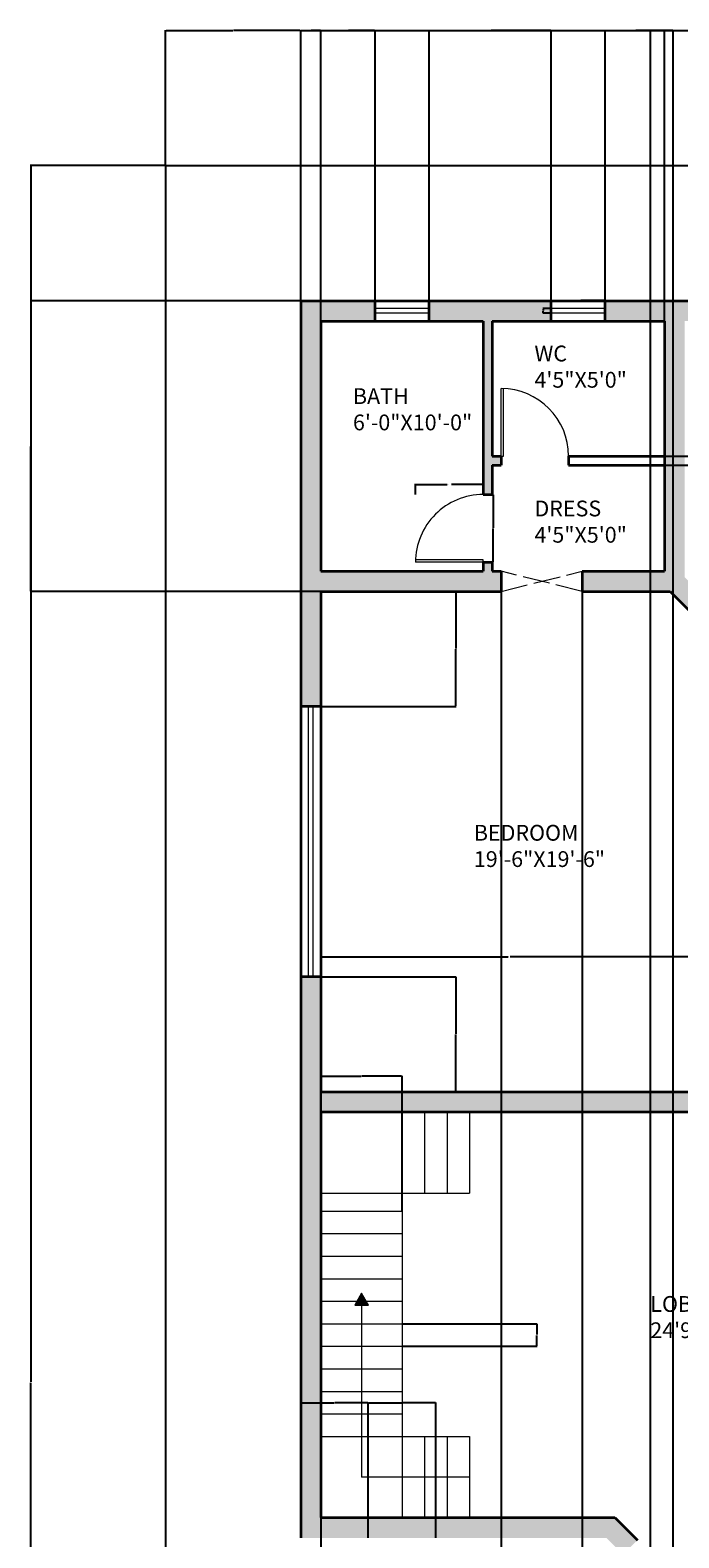
# Model space of a CAD drawing. Units: inches. Extents: x 1516 to 2236, y 3034 to 4235.
# Tile 2 of 3: x 1516 to 1804, y 3566 to 4235. Entities that reach past the tile are written whole.
import ezdxf

# ---------------------------------------------------------------- set-up
doc = ezdxf.new("R2010")
doc.units = ezdxf.units.IN
doc.linetypes.add('ACAD_ISO02W100', pattern=[15, 12, -3])
for name, color, linetype, lineweight in [('A-ANNO-DIMS', 2, 'Continuous', 18), ('A-ANNO-SYMB', 7, 'Continuous', 18), ('A-AREA-IDEN', 7, 'Continuous', 18), ('A-DOOR', 3, 'Continuous', 18), ('A-FLOR-STRS', 7, 'Continuous', 18), ('A-GLAZ', 4, 'Continuous', 18), ('A-WALL', 7, 'Continuous', 35), ('A-WALL-OVHD', 8, 'ACAD_ISO02W100', 13), ('A-WALL-PATT', 252, 'Continuous', 13), ('C-PROP', 8, 'Continuous', 25)]:
    doc.layers.add(name, color=color, linetype=linetype, lineweight=lineweight)
doc.styles.get("Standard").update_dxf_attribs({"font": 'arial.ttf'})
doc.dimstyles.get("Standard").update_dxf_attribs({"dimtxt": 0.18, "dimasz": 0.18, "dimexe": 0.18, "dimexo": 0.0625, "dimgap": 0.09, "dimtad": 0, "dimtih": 1, "dimtoh": 1, "dimdec": 4, "dimzin": 0, "dimdsep": 46, "dimtxsty": 'Standard', "dimcen": 0.09, "dimadec": 0, "dimazin": 0, "dimtfac": 1, "dimtdec": 4, "dimtofl": 0, "dimtmove": 0, "dimatfit": 3, "dimfxl": 1, "dimtolj": 1, "dimtzin": 0, "dimarcsym": 0})

# ---------------------------------------------------------------- blocks, each defined once
blk = doc.blocks.new('DOOR-30IN-SWING')
for p, q in [((0, 0), (0, 30)), ((1, 0), (1, 29.98)), ((0, 0), (1, 0))]:
    blk.add_line(p, q)
blk.add_arc((0, 0), 30, 0, 90)
blk = doc.blocks.new('WIN-120IN-GLASS')
for p, q in [((120, 2), (0, 2)), ((120, 0), (0, 0))]:
    blk.add_line(p, q)
blk = doc.blocks.new('WIN-24IN-GLASS')
for p, q in [((24, 2), (0, 2)), ((24, 0), (0, 0))]:
    blk.add_line(p, q)
blk = doc.blocks.new('*D8')
at = {"layer": 'A-ANNO-DIMS', "color": 0, "lineweight": -2, "transparency": 16777216}
for p, q in [((1747.26, 4111.08), (1747.26, 4114.8)), ((1747.44, 4114.62), (1758.15, 4114.62)), ((1771.08, 4114.62), (1760.38, 4114.62)), ((1771.26, 4111.08), (1771.26, 4114.8))]:
    blk.add_line(p, q, dxfattribs=at)
at = {"layer": 'A-ANNO-DIMS', "color": 0, "transparency": 16777216}
for points in [[(1747.44, 4114.65), (1747.44, 4114.59), (1747.26, 4114.62)], [(1771.08, 4114.65), (1771.08, 4114.59), (1771.26, 4114.62)]]:
    blk.add_solid(points, dxfattribs=at)
at = {"layer": 'Defpoints', "color": 0, "transparency": 16777216}
for p in [(1747.26, 4111.02), (1771.26, 4114.62), (1771.26, 4111.02)]:
    blk.add_point(p, dxfattribs=at)
at = {"layer": 'A-ANNO-DIMS', "color": 0, "transparency": 16777216, "insert": (1759.26, 4114.62), "char_height": 0.18, "attachment_point": 5}
blk.add_mtext('\\A1;WINDOW 24 TYP.', dxfattribs=at)
blk = doc.blocks.new('*D9')
at = {"layer": 'A-ANNO-DIMS', "color": 0, "lineweight": -2, "transparency": 16777216}
for p, q in [((1747.2, 4111.02), (1743.48, 4111.02)), ((1747.2, 4109.02), (1743.48, 4109.02)), ((1743.66, 4110.84), (1743.66, 4110.2)), ((1743.66, 4109.2), (1743.66, 4109.84))]:
    blk.add_line(p, q, dxfattribs=at)
at = {"layer": 'A-ANNO-DIMS', "color": 0, "transparency": 16777216}
for points in [[(1743.63, 4110.84), (1743.69, 4110.84), (1743.66, 4111.02)], [(1743.63, 4109.2), (1743.69, 4109.2), (1743.66, 4109.02)]]:
    blk.add_solid(points, dxfattribs=at)
at = {"layer": 'Defpoints', "color": 0, "transparency": 16777216}
for p in [(1743.66, 4111.02), (1747.26, 4111.02), (1747.26, 4109.02)]:
    blk.add_point(p, dxfattribs=at)
at = {"layer": 'A-ANNO-DIMS', "color": 0, "transparency": 16777216, "insert": (1743.66, 4110.02), "char_height": 0.18, "attachment_point": 5}
blk.add_mtext('\\A1;2 TYP.', dxfattribs=at)
blk = doc.blocks.new('*D14')
at = {"layer": 'A-ANNO-DIMS', "color": 0, "lineweight": -2, "transparency": 16777216}
for p, q in [((1687.01, 4028.58), (1687.01, 4033.2)), ((1687.19, 4033.02), (1701.08, 4033.02)), ((1716.83, 4033.02), (1702.95, 4033.02)), ((1717.01, 4028.58), (1717.01, 4033.2))]:
    blk.add_line(p, q, dxfattribs=at)
at = {"layer": 'A-ANNO-DIMS', "color": 0, "transparency": 16777216}
for points in [[(1687.19, 4033.05), (1687.19, 4032.99), (1687.01, 4033.02)], [(1716.83, 4033.05), (1716.83, 4032.99), (1717.01, 4033.02)]]:
    blk.add_solid(points, dxfattribs=at)
at = {"layer": 'Defpoints', "color": 0, "transparency": 16777216}
for p in [(1687.01, 4033.02), (1687.01, 4028.52), (1717.01, 4028.52)]:
    blk.add_point(p, dxfattribs=at)
at = {"layer": 'A-ANNO-DIMS', "color": 0, "transparency": 16777216, "insert": (1702.01, 4033.02), "char_height": 0.18, "attachment_point": 5}
blk.add_mtext('\\A1;DOOR 30 TYP.', dxfattribs=at)
blk = doc.blocks.new('*D15')
at = {"layer": 'A-ANNO-DIMS', "color": 0, "lineweight": -2, "transparency": 16777216}
for p, q in [((1717.08, 4028.52), (1721.69, 4028.52)), ((1721.51, 4028.34), (1721.51, 4013.7)), ((1721.51, 3998.7), (1721.51, 4013.34)), ((1717.08, 3998.52), (1721.69, 3998.52))]:
    blk.add_line(p, q, dxfattribs=at)
at = {"layer": 'A-ANNO-DIMS', "color": 0, "transparency": 16777216}
for points in [[(1721.48, 4028.34), (1721.54, 4028.34), (1721.51, 4028.52)], [(1721.48, 3998.7), (1721.54, 3998.7), (1721.51, 3998.52)]]:
    blk.add_solid(points, dxfattribs=at)
at = {"layer": 'Defpoints', "color": 0, "transparency": 16777216}
for p in [(1717.01, 4028.52), (1721.51, 4028.52), (1717.01, 3998.52)]:
    blk.add_point(p, dxfattribs=at)
at = {"layer": 'A-ANNO-DIMS', "color": 0, "transparency": 16777216, "insert": (1721.51, 4013.52), "char_height": 0.18, "attachment_point": 5}
blk.add_mtext('\\A1;30 TYP.', dxfattribs=at)
blk = doc.blocks.new('*D17')
at = {"layer": 'A-ANNO-DIMS', "color": 0, "lineweight": -2, "transparency": 16777216}
for p, q in [((1575.95, 4174.52), (1515.93, 4174.52)), ((1516.11, 4174.34), (1516.11, 3634.7)), ((1516.11, 3094.7), (1516.11, 3634.34)), ((1575.95, 3094.52), (1515.93, 3094.52))]:
    blk.add_line(p, q, dxfattribs=at)
at = {"layer": 'A-ANNO-DIMS', "color": 0, "transparency": 16777216}
for points in [[(1516.08, 4174.34), (1516.14, 4174.34), (1516.11, 4174.52)], [(1516.08, 3094.7), (1516.14, 3094.7), (1516.11, 3094.52)]]:
    blk.add_solid(points, dxfattribs=at)
at = {"layer": 'Defpoints', "color": 0, "transparency": 16777216}
for p in [(1516.11, 4174.52), (1576.01, 4174.52), (1576.01, 3094.52)]:
    blk.add_point(p, dxfattribs=at)
at = {"layer": 'A-ANNO-DIMS', "color": 0, "transparency": 16777216, "insert": (1516.11, 3634.52), "char_height": 0.18, "attachment_point": 5}
blk.add_mtext('\\A1;1080', dxfattribs=at)
blk = doc.blocks.new('*D18')
at = {"layer": 'A-ANNO-DIMS', "color": 0, "lineweight": -2, "transparency": 16777216}
for p, q in [((1576.01, 4174.58), (1576.01, 4234.6)), ((1576.19, 4234.42), (1605.8, 4234.42)), ((1635.83, 4234.42), (1606.23, 4234.42)), ((1636.01, 4114.58), (1636.01, 4234.6))]:
    blk.add_line(p, q, dxfattribs=at)
at = {"layer": 'A-ANNO-DIMS', "color": 0, "transparency": 16777216}
for points in [[(1576.19, 4234.45), (1576.19, 4234.39), (1576.01, 4234.42)], [(1635.83, 4234.45), (1635.83, 4234.39), (1636.01, 4234.42)]]:
    blk.add_solid(points, dxfattribs=at)
at = {"layer": 'Defpoints', "color": 0, "transparency": 16777216}
for p in [(1636.01, 4234.42), (1576.01, 4174.52), (1636.01, 4114.52)]:
    blk.add_point(p, dxfattribs=at)
at = {"layer": 'A-ANNO-DIMS', "color": 0, "transparency": 16777216, "insert": (1606.01, 4234.42), "char_height": 0.18, "attachment_point": 5}
blk.add_mtext('\\A1;60', dxfattribs=at)
blk = doc.blocks.new('*D19')
at = {"layer": 'A-ANNO-DIMS', "color": 0, "lineweight": -2, "transparency": 16777216}
for p, q in [((1636.01, 4114.58), (1636.01, 4234.6)), ((1636.19, 4234.42), (1875.37, 4234.42)), ((2115.33, 4234.42), (1876.16, 4234.42)), ((2115.51, 4114.58), (2115.51, 4234.6))]:
    blk.add_line(p, q, dxfattribs=at)
at = {"layer": 'A-ANNO-DIMS', "color": 0, "transparency": 16777216}
for points in [[(1636.19, 4234.45), (1636.19, 4234.39), (1636.01, 4234.42)], [(2115.33, 4234.45), (2115.33, 4234.39), (2115.51, 4234.42)]]:
    blk.add_solid(points, dxfattribs=at)
at = {"layer": 'Defpoints', "color": 0, "transparency": 16777216}
for p in [(2115.51, 4234.42), (1636.01, 4114.52), (2115.51, 4114.52)]:
    blk.add_point(p, dxfattribs=at)
at = {"layer": 'A-ANNO-DIMS', "color": 0, "transparency": 16777216, "insert": (1875.76, 4234.42), "char_height": 0.18, "attachment_point": 5}
blk.add_mtext('\\A1;479.5', dxfattribs=at)
blk = doc.blocks.new('*D29')
at = {"layer": 'A-ANNO-DIMS', "color": 0, "lineweight": -2, "transparency": 16777216}
for p, q in [((1645.08, 3985.52), (1705.09, 3985.52)), ((1704.91, 3985.34), (1704.91, 3960.2)), ((1704.91, 3934.7), (1704.91, 3959.84)), ((1645.08, 3934.52), (1705.09, 3934.52))]:
    blk.add_line(p, q, dxfattribs=at)
at = {"layer": 'A-ANNO-DIMS', "color": 0, "transparency": 16777216}
for points in [[(1704.88, 3985.34), (1704.94, 3985.34), (1704.91, 3985.52)], [(1704.88, 3934.7), (1704.94, 3934.7), (1704.91, 3934.52)]]:
    blk.add_solid(points, dxfattribs=at)
at = {"layer": 'Defpoints', "color": 0, "transparency": 16777216}
for p in [(1645.01, 3985.52), (1645.01, 3934.52), (1704.91, 3934.52)]:
    blk.add_point(p, dxfattribs=at)
at = {"layer": 'A-ANNO-DIMS', "color": 0, "transparency": 16777216, "insert": (1704.91, 3960.02), "char_height": 0.18, "attachment_point": 5}
blk.add_mtext('\\A1;51', dxfattribs=at)
blk = doc.blocks.new('*D30')
at = {"layer": 'A-ANNO-DIMS', "color": 0, "lineweight": -2, "transparency": 16777216}
for p, q in [((1645.08, 3814.52), (1705.09, 3814.52)), ((1704.91, 3814.34), (1704.91, 3789.2)), ((1704.91, 3763.7), (1704.91, 3788.84)), ((1645.08, 3763.52), (1705.09, 3763.52))]:
    blk.add_line(p, q, dxfattribs=at)
at = {"layer": 'A-ANNO-DIMS', "color": 0, "transparency": 16777216}
for points in [[(1704.88, 3814.34), (1704.94, 3814.34), (1704.91, 3814.52)], [(1704.88, 3763.7), (1704.94, 3763.7), (1704.91, 3763.52)]]:
    blk.add_solid(points, dxfattribs=at)
at = {"layer": 'Defpoints', "color": 0, "transparency": 16777216}
for p in [(1645.01, 3814.52), (1645.01, 3763.52), (1704.91, 3763.52)]:
    blk.add_point(p, dxfattribs=at)
at = {"layer": 'A-ANNO-DIMS', "color": 0, "transparency": 16777216, "insert": (1704.91, 3789.02), "char_height": 0.18, "attachment_point": 5}
blk.add_mtext('\\A1;51', dxfattribs=at)
blk = doc.blocks.new('*D31')
at = {"layer": 'A-ANNO-DIMS', "color": 0, "lineweight": -2, "transparency": 16777216}
for p, q in [((1645.01, 3763.58), (1645.01, 3823.6)), ((1645.19, 3823.42), (1728.13, 3823.42)), ((1811.97, 3823.42), (1729.04, 3823.42)), ((1812.15, 3763.58), (1812.15, 3823.6))]:
    blk.add_line(p, q, dxfattribs=at)
at = {"layer": 'A-ANNO-DIMS', "color": 0, "transparency": 16777216}
for points in [[(1645.19, 3823.45), (1645.19, 3823.39), (1645.01, 3823.42)], [(1811.97, 3823.45), (1811.97, 3823.39), (1812.15, 3823.42)]]:
    blk.add_solid(points, dxfattribs=at)
at = {"layer": 'Defpoints', "color": 0, "transparency": 16777216}
for p in [(1812.15, 3823.42), (1645.01, 3763.52), (1812.15, 3763.52)]:
    blk.add_point(p, dxfattribs=at)
at = {"layer": 'A-ANNO-DIMS', "color": 0, "transparency": 16777216, "insert": (1728.58, 3823.42), "char_height": 0.18, "attachment_point": 5}
blk.add_mtext('\\A1;167.14', dxfattribs=at)
blk = doc.blocks.new('*D32')
at = {"layer": 'A-ANNO-DIMS', "color": 0, "lineweight": -2, "transparency": 16777216}
for p, q in [((1636.01, 3565.58), (1636.01, 3625.6)), ((1636.19, 3625.42), (1650.8, 3625.42)), ((1665.83, 3625.42), (1651.23, 3625.42)), ((1666.01, 3565.58), (1666.01, 3625.6))]:
    blk.add_line(p, q, dxfattribs=at)
at = {"layer": 'A-ANNO-DIMS', "color": 0, "transparency": 16777216}
for points in [[(1636.19, 3625.45), (1636.19, 3625.39), (1636.01, 3625.42)], [(1665.83, 3625.45), (1665.83, 3625.39), (1666.01, 3625.42)]]:
    blk.add_solid(points, dxfattribs=at)
at = {"layer": 'Defpoints', "color": 0, "transparency": 16777216}
for p in [(1666.01, 3625.42), (1636.01, 3565.52), (1666.01, 3565.52)]:
    blk.add_point(p, dxfattribs=at)
at = {"layer": 'A-ANNO-DIMS', "color": 0, "transparency": 16777216, "insert": (1651.01, 3625.42), "char_height": 0.18, "attachment_point": 5}
blk.add_mtext('\\A1;30', dxfattribs=at)
blk = doc.blocks.new('*D33')
at = {"layer": 'A-ANNO-DIMS', "color": 0, "lineweight": -2, "transparency": 16777216}
for p, q in [((1666.01, 3565.58), (1666.01, 3625.6)), ((1666.19, 3625.42), (1680.8, 3625.42)), ((1695.83, 3625.42), (1681.23, 3625.42)), ((1696.01, 3565.58), (1696.01, 3625.6))]:
    blk.add_line(p, q, dxfattribs=at)
at = {"layer": 'A-ANNO-DIMS', "color": 0, "transparency": 16777216}
for points in [[(1666.19, 3625.45), (1666.19, 3625.39), (1666.01, 3625.42)], [(1695.83, 3625.45), (1695.83, 3625.39), (1696.01, 3625.42)]]:
    blk.add_solid(points, dxfattribs=at)
at = {"layer": 'Defpoints', "color": 0, "transparency": 16777216}
for p in [(1696.01, 3625.42), (1666.01, 3565.52), (1696.01, 3565.52)]:
    blk.add_point(p, dxfattribs=at)
at = {"layer": 'A-ANNO-DIMS', "color": 0, "transparency": 16777216, "insert": (1681.01, 3625.42), "char_height": 0.18, "attachment_point": 5}
blk.add_mtext('\\A1;30', dxfattribs=at)
blk = doc.blocks.new('*D34')
at = {"layer": 'A-ANNO-DIMS', "color": 0, "lineweight": -2, "transparency": 16777216}
for p, q in [((1645.01, 4105.58), (1645.01, 4234.6)), ((1645.19, 4234.42), (1656.79, 4234.42)), ((1668.83, 4234.42), (1657.23, 4234.42)), ((1669.01, 4114.58), (1669.01, 4234.6))]:
    blk.add_line(p, q, dxfattribs=at)
at = {"layer": 'A-ANNO-DIMS', "color": 0, "transparency": 16777216}
for points in [[(1645.19, 4234.45), (1645.19, 4234.39), (1645.01, 4234.42)], [(1668.83, 4234.45), (1668.83, 4234.39), (1669.01, 4234.42)]]:
    blk.add_solid(points, dxfattribs=at)
at = {"layer": 'Defpoints', "color": 0, "transparency": 16777216}
for p in [(1669.01, 4234.42), (1669.01, 4114.52), (1645.01, 4105.52)]:
    blk.add_point(p, dxfattribs=at)
at = {"layer": 'A-ANNO-DIMS', "color": 0, "transparency": 16777216, "insert": (1657.01, 4234.42), "char_height": 0.18, "attachment_point": 5}
blk.add_mtext('\\A1;24', dxfattribs=at)
blk = doc.blocks.new('*D35')
at = {"layer": 'A-ANNO-DIMS', "color": 0, "lineweight": -2, "transparency": 16777216}
for p, q in [((1693.01, 4114.58), (1693.01, 4234.6)), ((1693.19, 4234.42), (1719.74, 4234.42)), ((1747.08, 4234.42), (1720.53, 4234.42)), ((1747.26, 4114.58), (1747.26, 4234.6))]:
    blk.add_line(p, q, dxfattribs=at)
at = {"layer": 'A-ANNO-DIMS', "color": 0, "transparency": 16777216}
for points in [[(1693.19, 4234.45), (1693.19, 4234.39), (1693.01, 4234.42)], [(1747.08, 4234.45), (1747.08, 4234.39), (1747.26, 4234.42)]]:
    blk.add_solid(points, dxfattribs=at)
at = {"layer": 'Defpoints', "color": 0, "transparency": 16777216}
for p in [(1747.26, 4234.42), (1693.01, 4114.52), (1747.26, 4114.52)]:
    blk.add_point(p, dxfattribs=at)
at = {"layer": 'A-ANNO-DIMS', "color": 0, "transparency": 16777216, "insert": (1720.14, 4234.42), "char_height": 0.18, "attachment_point": 5}
blk.add_mtext('\\A1;54.25', dxfattribs=at)
blk = doc.blocks.new('*D36')
at = {"layer": 'A-ANNO-DIMS', "color": 0, "lineweight": -2, "transparency": 16777216}
for p, q in [((1771.26, 4114.58), (1771.26, 4234.6)), ((1771.44, 4234.42), (1783.99, 4234.42)), ((1797.33, 4234.42), (1784.79, 4234.42)), ((1797.51, 4105.58), (1797.51, 4234.6))]:
    blk.add_line(p, q, dxfattribs=at)
at = {"layer": 'A-ANNO-DIMS', "color": 0, "transparency": 16777216}
for points in [[(1771.44, 4234.45), (1771.44, 4234.39), (1771.26, 4234.42)], [(1797.33, 4234.45), (1797.33, 4234.39), (1797.51, 4234.42)]]:
    blk.add_solid(points, dxfattribs=at)
at = {"layer": 'Defpoints', "color": 0, "transparency": 16777216}
for p in [(1797.51, 4234.42), (1771.26, 4114.52), (1797.51, 4105.52)]:
    blk.add_point(p, dxfattribs=at)
at = {"layer": 'A-ANNO-DIMS', "color": 0, "transparency": 16777216, "insert": (1784.39, 4234.42), "char_height": 0.18, "attachment_point": 5}
blk.add_mtext('\\A1;26.25', dxfattribs=at)
blk = doc.blocks.new('*D37')
at = {"layer": 'A-ANNO-DIMS', "color": 0, "lineweight": -2, "transparency": 16777216}
for p, q in [((1645.01, 3985.46), (1645.01, 3034.44)), ((1725.01, 3985.46), (1725.01, 3034.44)), ((1645.19, 3034.62), (1684.8, 3034.62)), ((1724.83, 3034.62), (1685.23, 3034.62))]:
    blk.add_line(p, q, dxfattribs=at)
at = {"layer": 'A-ANNO-DIMS', "color": 0, "transparency": 16777216}
for points in [[(1645.19, 3034.65), (1645.19, 3034.59), (1645.01, 3034.62)], [(1724.83, 3034.65), (1724.83, 3034.59), (1725.01, 3034.62)]]:
    blk.add_solid(points, dxfattribs=at)
at = {"layer": 'Defpoints', "color": 0, "transparency": 16777216}
for p in [(1645.01, 3985.52), (1725.01, 3985.52), (1725.01, 3034.62)]:
    blk.add_point(p, dxfattribs=at)
at = {"layer": 'A-ANNO-DIMS', "color": 0, "transparency": 16777216, "insert": (1685.01, 3034.62), "char_height": 0.18, "attachment_point": 5}
blk.add_mtext('\\A1;80', dxfattribs=at)
blk = doc.blocks.new('*D38')
at = {"layer": 'A-ANNO-DIMS', "color": 0, "lineweight": -2, "transparency": 16777216}
for p, q in [((1725.01, 3985.46), (1725.01, 3034.44)), ((1761.01, 3985.46), (1761.01, 3034.44)), ((1725.19, 3034.62), (1742.8, 3034.62)), ((1760.83, 3034.62), (1743.23, 3034.62))]:
    blk.add_line(p, q, dxfattribs=at)
at = {"layer": 'A-ANNO-DIMS', "color": 0, "transparency": 16777216}
for points in [[(1725.19, 3034.65), (1725.19, 3034.59), (1725.01, 3034.62)], [(1760.83, 3034.65), (1760.83, 3034.59), (1761.01, 3034.62)]]:
    blk.add_solid(points, dxfattribs=at)
at = {"layer": 'Defpoints', "color": 0, "transparency": 16777216}
for p in [(1725.01, 3985.52), (1761.01, 3985.52), (1761.01, 3034.62)]:
    blk.add_point(p, dxfattribs=at)
at = {"layer": 'A-ANNO-DIMS', "color": 0, "transparency": 16777216, "insert": (1743.01, 3034.62), "char_height": 0.18, "attachment_point": 5}
blk.add_mtext('\\A1;36', dxfattribs=at)
blk = doc.blocks.new('*D39')
at = {"layer": 'A-ANNO-DIMS', "color": 0, "lineweight": -2, "transparency": 16777216}
for p, q in [((1797.57679, 4045.522053), (2236.09429, 4045.522053)), ((1797.57679, 4041.522053), (2236.09429, 4041.522053)), ((2235.91429, 4045.342053), (2235.91429, 4043.702053)), ((2235.91429, 4041.702053), (2235.91429, 4043.342053))]:
    blk.add_line(p, q, dxfattribs=at)
at = {"layer": 'A-ANNO-DIMS', "color": 0, "transparency": 16777216}
for points in [[(2235.88429, 4045.342053), (2235.94429, 4045.342053), (2235.91429, 4045.522053)], [(2235.88429, 4041.702053), (2235.94429, 4041.702053), (2235.91429, 4041.522053)]]:
    blk.add_solid(points, dxfattribs=at)
at = {"layer": 'Defpoints', "color": 0, "transparency": 16777216}
for p in [(1797.51429, 4045.522053), (1797.51429, 4041.522053), (2235.91429, 4045.522053)]:
    blk.add_point(p, dxfattribs=at)
at = {"layer": 'A-ANNO-DIMS', "color": 0, "transparency": 16777216, "insert": (2235.91429, 4043.522053), "char_height": 0.18, "attachment_point": 5}
blk.add_mtext('\\A1;4', dxfattribs=at)
blk = doc.blocks.new('*D40')
at = {"layer": 'A-ANNO-DIMS', "color": 0, "lineweight": -2, "transparency": 16777216}
for p, q in [((1635.95, 4114.52), (1515.93, 4114.52)), ((1516.11, 4114.34), (1516.11, 4050.2)), ((1516.11, 3985.7), (1516.11, 4049.84)), ((1644.95, 3985.52), (1515.93, 3985.52))]:
    blk.add_line(p, q, dxfattribs=at)
at = {"layer": 'A-ANNO-DIMS', "color": 0, "transparency": 16777216}
for points in [[(1516.08, 4114.34), (1516.14, 4114.34), (1516.11, 4114.52)], [(1516.08, 3985.7), (1516.14, 3985.7), (1516.11, 3985.52)]]:
    blk.add_solid(points, dxfattribs=at)
at = {"layer": 'Defpoints', "color": 0, "transparency": 16777216}
for p in [(1636.01, 4114.52), (1516.11, 3985.52), (1645.01, 3985.52)]:
    blk.add_point(p, dxfattribs=at)
at = {"layer": 'A-ANNO-DIMS', "color": 0, "transparency": 16777216, "insert": (1516.11, 4050.02), "char_height": 0.18, "attachment_point": 5}
blk.add_mtext('\\A1;129', dxfattribs=at)
blk = doc.blocks.new('*D41')
at = {"layer": 'A-ANNO-DIMS', "color": 0, "lineweight": -2, "transparency": 16777216}
for p, q in [((1636.01, 4114.58), (1636.01, 4234.6)), ((1636.19, 4234.42), (1640.37, 4234.42)), ((1644.83, 4234.42), (1640.66, 4234.42)), ((1645.01, 4105.58), (1645.01, 4234.6))]:
    blk.add_line(p, q, dxfattribs=at)
at = {"layer": 'A-ANNO-DIMS', "color": 0, "transparency": 16777216}
for points in [[(1636.19, 4234.45), (1636.19, 4234.39), (1636.01, 4234.42)], [(1644.83, 4234.45), (1644.83, 4234.39), (1645.01, 4234.42)]]:
    blk.add_solid(points, dxfattribs=at)
at = {"layer": 'Defpoints', "color": 0, "transparency": 16777216}
for p in [(1645.01, 4234.42), (1636.01, 4114.52), (1645.01, 4105.52)]:
    blk.add_point(p, dxfattribs=at)
at = {"layer": 'A-ANNO-DIMS', "color": 0, "transparency": 16777216, "insert": (1640.51, 4234.42), "char_height": 0.18, "attachment_point": 5}
blk.add_mtext('\\A1;9', dxfattribs=at)
blk = doc.blocks.new('*D49')
at = {"layer": 'A-ANNO-DIMS', "color": 0, "lineweight": -2, "transparency": 16777216}
for p, q in [((1791.4, 3240.97), (1791.4, 4234.6)), ((1791.58, 4234.42), (1796.19, 4234.42)), ((1801.22, 4234.42), (1796.61, 4234.42)), ((1801.4, 3240.97), (1801.4, 4234.6))]:
    blk.add_line(p, q, dxfattribs=at)
at = {"layer": 'A-ANNO-DIMS', "color": 0, "transparency": 16777216}
for points in [[(1791.58, 4234.45), (1791.58, 4234.39), (1791.4, 4234.42)], [(1801.22, 4234.45), (1801.22, 4234.39), (1801.4, 4234.42)]]:
    blk.add_solid(points, dxfattribs=at)
at = {"layer": 'Defpoints', "color": 0, "transparency": 16777216}
for p in [(1801.4, 4234.42), (1791.4, 3240.91), (1801.4, 3240.91)]:
    blk.add_point(p, dxfattribs=at)
at = {"layer": 'A-ANNO-DIMS', "color": 0, "transparency": 16777216, "insert": (1796.4, 4234.42), "char_height": 0.18, "attachment_point": 5}
blk.add_mtext('\\A1;10', dxfattribs=at)
blk = doc.blocks.new('*D54')
at = {"layer": 'A-ANNO-DIMS', "color": 0, "lineweight": -2, "transparency": 16777216}
for p, q in [((1645.01, 3710.58), (1645.01, 3770.6)), ((1645.19, 3770.42), (1662.8, 3770.42)), ((1680.83, 3770.42), (1663.23, 3770.42)), ((1681.01, 3710.58), (1681.01, 3770.6))]:
    blk.add_line(p, q, dxfattribs=at)
at = {"layer": 'A-ANNO-DIMS', "color": 0, "transparency": 16777216}
for points in [[(1645.19, 3770.45), (1645.19, 3770.39), (1645.01, 3770.42)], [(1680.83, 3770.45), (1680.83, 3770.39), (1681.01, 3770.42)]]:
    blk.add_solid(points, dxfattribs=at)
at = {"layer": 'Defpoints', "color": 0, "transparency": 16777216}
for p in [(1681.01, 3770.42), (1645.01, 3710.52), (1681.01, 3710.52)]:
    blk.add_point(p, dxfattribs=at)
at = {"layer": 'A-ANNO-DIMS', "color": 0, "transparency": 16777216, "insert": (1663.01, 3770.42), "char_height": 0.18, "attachment_point": 5}
blk.add_mtext('\\A1;36', dxfattribs=at)
blk = doc.blocks.new('*D55')
at = {"layer": 'A-ANNO-DIMS', "color": 0, "lineweight": -2, "transparency": 16777216}
for p, q in [((1681.08, 3660.52), (1741.09, 3660.52)), ((1740.91, 3660.34), (1740.91, 3655.7)), ((1740.91, 3650.7), (1740.91, 3655.34)), ((1681.08, 3650.52), (1741.09, 3650.52))]:
    blk.add_line(p, q, dxfattribs=at)
at = {"layer": 'A-ANNO-DIMS', "color": 0, "transparency": 16777216}
for points in [[(1740.88, 3660.34), (1740.94, 3660.34), (1740.91, 3660.52)], [(1740.88, 3650.7), (1740.94, 3650.7), (1740.91, 3650.52)]]:
    blk.add_solid(points, dxfattribs=at)
at = {"layer": 'Defpoints', "color": 0, "transparency": 16777216}
for p in [(1681.01, 3660.52), (1681.01, 3650.52), (1740.91, 3650.52)]:
    blk.add_point(p, dxfattribs=at)
at = {"layer": 'A-ANNO-DIMS', "color": 0, "transparency": 16777216, "insert": (1740.91, 3655.52), "char_height": 0.18, "attachment_point": 5}
blk.add_mtext('\\A1;10', dxfattribs=at)

msp = doc.modelspace()

# ---------------------------------------------------------------- hatches: boundary and pattern name
at = {"layer": 'A-ANNO-SYMB'}
h = msp.add_hatch(color=256, dxfattribs=at)
h.dxf.hatch_style = 1
h.paths.add_polyline_path([(1663.0143, 3674.0323), (1659.9743, 3668.7669), (1666.0542, 3668.7669)])
at = {"layer": 'A-WALL-PATT'}
h = msp.add_hatch(color=256, dxfattribs=at)
h.dxf.hatch_style = 1
h.paths.add_polyline_path([(2115.5143, 3444.4097), (2106.5143, 3444.4097), (2106.5143, 3372.4097), (1977.6285, 3372.4097), (1845.6285, 3504.4097), (1862.599, 3521.3803), (1856.2351, 3527.7442), (1839.2645, 3510.7737), (1836.4361, 3513.6021), (1830.0721, 3507.2381), (1973.9005, 3363.4097), (2115.5143, 3363.4097)])
h.paths.add_polyline_path([(2115.5143, 3671.9887), (2106.5143, 3671.9887), (2106.5143, 3645.4097), (1981.3564, 3645.4097), (1963.6205, 3663.1456), (1957.2565, 3656.7817), (1971.2645, 3642.7737), (1954.2939, 3625.8031), (1960.6579, 3619.4391), (1977.6285, 3636.4097), (2106.5143, 3636.4097), (2106.5143, 3564.4097), (2115.5143, 3564.4097)])
h.paths.add_polyline_path([(1975.583, 3914.2268), (1978.4114, 3917.0552), (1972.0475, 3923.4192), (1951.7986, 3903.1703), (1958.1625, 3896.8063), (1969.219, 3907.8629), (2030.7373, 3846.3446), (1905.5794, 3721.1867), (1901.3368, 3725.4293), (1894.9728, 3719.0653), (1923.3154, 3690.7228), (1929.6793, 3697.0868), (1911.9434, 3714.8227), (2037.1013, 3839.9806), (2106.5143, 3770.5676), (2106.5143, 3743.9887), (2115.5143, 3743.9887), (2115.5143, 3774.2955), (2056.9238, 3832.886), (2115.5143, 3891.4765), (2115.5143, 3928.3632), (2106.5143, 3928.3632), (2106.5143, 3895.2044), (2050.5598, 3839.25)])
h.paths.add_polyline_path([(1806.5143, 3991.886), (1806.5143, 4105.5221), (1863.5143, 4105.5221), (1863.5143, 4114.5221), (1771.2643, 4114.5221), (1771.2643, 4105.5221), (1797.5143, 4105.5221), (1797.5143, 3994.5221), (1761.0143, 3994.5221), (1761.0143, 3985.5221), (1800.1503, 3985.5221), (1917.1503, 3868.5221), (1914.3219, 3865.6936), (1920.6859, 3859.3297), (1923.5143, 3862.1581), (1932.7067, 3871.3505), (1926.3427, 3877.7144), (1923.5143, 3874.886)])
h.paths.add_polyline_path([(1895.23, 3833.8738), (1888.8661, 3840.2378), (1812.1503, 3763.5221), (1645.0143, 3763.5221), (1645.0143, 3814.5221), (1636.0143, 3814.5221), (1636.0143, 3565.5221), (1771.7882, 3565.5221), (1779.1604, 3558.1498), (1785.5244, 3564.5138), (1775.5161, 3574.5221), (1645.0143, 3574.5221), (1645.0143, 3754.5221), (1815.8783, 3754.5221), (1837.6972, 3776.341), (1841.9398, 3772.0983), (1848.3038, 3778.4623), (1844.0611, 3782.7049)])
h.paths.add_polyline_path([(1645.0143, 3985.5221), (1725.0143, 3985.5221), (1725.0143, 3994.5221), (1721.0143, 3994.5221), (1721.0143, 3998.5221), (1717.0143, 3998.5221), (1717.0143, 3994.5221), (1645.0143, 3994.5221), (1645.0143, 4105.5221), (1669.0143, 4105.5221), (1669.0143, 4114.5221), (1636.0143, 4114.5221), (1636.0143, 3934.5221), (1645.0143, 3934.5221)])
h.paths.add_polyline_path([(1747.2643, 4114.5221), (1693.0143, 4114.5221), (1693.0143, 4105.5221), (1717.0143, 4105.5221), (1717.0143, 4028.5221), (1721.0143, 4028.5221), (1721.0143, 4041.5221), (1725.0143, 4041.5221), (1725.0143, 4045.5221), (1721.0143, 4045.5221), (1721.0143, 4105.5221), (1747.2643, 4105.5221)])
h.paths.add_polyline_path([(2066.0143, 4114.5221), (1983.5143, 4114.5221), (1983.5143, 4105.5221), (2040.5143, 4105.5221), (2040.5143, 4068.0221), (2049.5143, 4068.0221), (2049.5143, 4105.5221), (2066.0143, 4105.5221)])
h.paths.add_polyline_path([(2115.5143, 4114.5221), (2090.0143, 4114.5221), (2090.0143, 4105.5221), (2106.5143, 4105.5221), (2106.5143, 3994.5221), (2049.5143, 3994.5221), (2049.5143, 4032.0221), (2040.5143, 4032.0221), (2040.5143, 3991.886), (1997.5033, 3948.875), (2003.8673, 3942.5111), (2046.8783, 3985.5221), (2106.5143, 3985.5221), (2106.5143, 3952.3632), (2115.5143, 3952.3632)])
h.paths.add_polyline_path([(1789.2236, 3395.8151), (1636.0143, 3395.8151), (1636.0143, 3386.8151), (1785.4957, 3386.8151), (1891.4008, 3280.91), (1897.7648, 3287.2739)])

# ---------------------------------------------------------------- linework, layer by layer
at = {"layer": 'A-ANNO-SYMB'}
for p in [(1663.0143, 3668.7669), (1711.0143, 3592.5221)]:
    msp.add_line(p, (1663.0143, 3592.5221), dxfattribs=at)
msp.add_lwpolyline([(1663.0143, 3674.0323), (1659.9743, 3668.7669), (1666.0542, 3668.7669)], close=True, dxfattribs=at)
at = {"layer": 'A-FLOR-STRS'}
for p, q in [((1681.0143, 3754.5221), (1681.0143, 3574.5221)), ((1691.0143, 3754.5221), (1691.0143, 3718.5221)), ((1701.0143, 3754.5221), (1701.0143, 3718.5221)), ((1711.0143, 3754.5221), (1711.0143, 3718.5221)), ((1645.0143, 3718.5221), (1711.0143, 3718.5221)), ((1645.0143, 3710.5221), (1681.0143, 3710.5221)), ((1645.0143, 3700.5221), (1681.0143, 3700.5221)), ((1645.0143, 3690.5221), (1681.0143, 3690.5221)), ((1645.0143, 3680.5221), (1681.0143, 3680.5221)), ((1645.0143, 3670.5221), (1660.9877, 3670.5221)), ((1665.0409, 3670.5221), (1681.0143, 3670.5221)), ((1645.0143, 3660.5221), (1681.0143, 3660.5221)), ((1645.0143, 3650.5221), (1681.0143, 3650.5221)), ((1645.0143, 3640.5221), (1681.0143, 3640.5221)), ((1645.0143, 3630.5221), (1681.0143, 3630.5221)), ((1645.0143, 3620.5221), (1681.0143, 3620.5221)), ((1645.0143, 3610.5221), (1711.0143, 3610.5221)), ((1691.0143, 3610.5221), (1691.0143, 3574.5221)), ((1701.0143, 3610.5221), (1701.0143, 3574.5221)), ((1711.0143, 3610.5221), (1711.0143, 3574.5221))]:
    msp.add_line(p, q, dxfattribs=at)
at = {"layer": 'A-WALL'}
for p, q in [((1636.0143, 4114.5221), (2115.5143, 4114.5221)), ((1636.0143, 4114.5221), (1636.0143, 3565.5221)), ((1669.0143, 4105.5221), (1669.0143, 4114.5221)), ((1693.0143, 4105.5221), (1693.0143, 4114.5221)), ((1747.2643, 4105.5221), (1747.2643, 4114.5221)), ((1771.2643, 4105.5221), (1771.2643, 4114.5221)), ((1645.0143, 4105.5221), (1717.0143, 4105.5221)), ((1645.0143, 4105.5221), (1645.0143, 3994.5221)), ((1717.0143, 4105.5221), (1717.0143, 4028.5221)), ((1721.0143, 4105.5221), (1721.0143, 4045.5221)), ((1721.0143, 4105.5221), (1797.5143, 4105.5221)), ((1797.5143, 4105.5221), (1797.5143, 3994.5221)), ((1721.0143, 4045.5221), (1725.0143, 4045.5221)), ((1721.0143, 4041.5221), (1725.0143, 4041.5221)), ((1721.0143, 4041.5221), (1721.0143, 4028.5221)), ((1725.0143, 4045.5221), (1725.0143, 4041.5221)), ((1755.0143, 4045.5221), (1755.0143, 4041.5221)), ((1755.0143, 4045.5221), (1797.5143, 4045.5221)), ((1755.0143, 4041.5221), (1797.5143, 4041.5221)), ((1717.0143, 4028.5221), (1721.0143, 4028.5221)), ((1645.0143, 3994.5221), (1717.0143, 3994.5221)), ((1717.0143, 3998.5221), (1721.0143, 3998.5221)), ((1717.0143, 3998.5221), (1717.0143, 3994.5221)), ((1721.0143, 3998.5221), (1721.0143, 3994.5221)), ((1721.0143, 3994.5221), (1725.0143, 3994.5221)), ((1725.0143, 3994.5221), (1725.0143, 3985.5221)), ((1761.0143, 3994.5221), (1761.0143, 3985.5221)), ((1761.0143, 3994.5221), (1797.5143, 3994.5221)), ((1645.0143, 3985.5221), (1725.0143, 3985.5221)), ((1645.0143, 3985.5221), (1645.0143, 3763.5221)), ((1761.0143, 3985.5221), (1800.1503, 3985.5221)), ((1800.1503, 3985.5221), (1917.1503, 3868.5221)), ((1645.0143, 3934.5221), (1636.0143, 3934.5221)), ((1645.0143, 3814.5221), (1636.0143, 3814.5221)), ((1645.0143, 3763.5221), (1812.1503, 3763.5221)), ((1645.0143, 3754.5221), (1815.8783, 3754.5221)), ((1645.0143, 3754.5221), (1645.0143, 3574.5221)), ((1645.0143, 3574.5221), (1775.5161, 3574.5221)), ((1775.5161, 3574.5221), (1785.5244, 3564.5138))]:
    msp.add_line(p, q, dxfattribs=at)
at = {"layer": 'A-WALL-OVHD'}
for p, q in [((1725.0143, 3985.5221), (1761.0143, 3994.5221)), ((1761.0143, 3985.5221), (1725.0143, 3994.5221))]:
    msp.add_line(p, q, dxfattribs=at)
at = {"layer": 'C-PROP'}
for q in [(2176.0143, 4174.5221), (1576.0143, 3094.5221)]:
    msp.add_line((1576.0143, 4174.5221), q, dxfattribs=at)

# ---------------------------------------------------------------- block references
at = {"layer": 'A-DOOR'}
msp.add_blockref('DOOR-30IN-SWING', (1725.0143, 4045.5221), dxfattribs=at)
at = {"layer": 'A-DOOR', "rotation": 89.99999999999834}
msp.add_blockref('DOOR-30IN-SWING', (1717.0143, 3998.5221), dxfattribs=at)
at = {"layer": 'A-GLAZ'}
for p in [(1669.0143, 4109.0221), (1747.2643, 4109.0221)]:
    msp.add_blockref('WIN-24IN-GLASS', p, dxfattribs=at)
at = {"layer": 'A-GLAZ', "rotation": 269.9999999999952}
msp.add_blockref('WIN-120IN-GLASS', (1639.5143, 3934.5221), dxfattribs=at)

# ---------------------------------------------------------------- texts
at = {"layer": 'A-AREA-IDEN', "char_height": 7, "attachment_point": 1}
for s, insert in [('WC\\P4\'5"X5\'0"', (1739.8184, 4094.6067)), ('BATH\\P6\'-0"X10\'-0"', (1659.2087, 4075.6927)), ('DRESS\\P4\'5"X5\'0"', (1739.8184, 4025.8265)), ('BEDROOM\\P19\'-6"X19\'-6"', (1712.9074, 3881.9119)), ('LOBBY\\P24\'9"X15\'0"', (1791.2759, 3672.8127))]:
    msp.add_mtext_dynamic_manual_height_columns(s, width=47.692137, gutter_width=12.5, heights=[0], dxfattribs=dict(at, insert=insert))

# ---------------------------------------------------------------- dimensions: what is measured, and where the dimension line sits
at = {"layer": 'A-ANNO-DIMS'}
for base, p1, p2, override, picture, middle in [((1636.0143, 4234.4221), (1576.0143, 4174.5221), (1636.0143, 4114.5221), {"dimdec": 0, "dimlfac": 1, "dimrnd": 0, "dimzin": 0, "dimdsep": 46, "dimlunit": 2}, '*D18', (1606.0143, 4234.4221)), ((2115.5143, 4234.4221), (1636.0143, 4114.5221), (2115.5143, 4114.5221), {"dimdec": 1, "dimlfac": 1, "dimrnd": 0, "dimzin": 0, "dimdsep": 46, "dimlunit": 2}, '*D19', (1875.7643, 4234.4221)), ((1645.0143, 4234.4221), (1636.0143, 4114.5221), (1645.0143, 4105.5221), {"dimdec": 0, "dimlfac": 1, "dimrnd": 0, "dimzin": 0, "dimdsep": 46, "dimlunit": 2}, '*D41', (1640.5143, 4234.4221)), ((1669.0143, 4234.4221), (1645.0143, 4105.5221), (1669.0143, 4114.5221), {"dimdec": 0, "dimlfac": 1, "dimrnd": 0, "dimzin": 0, "dimdsep": 46, "dimlunit": 2}, '*D34', (1657.0143, 4234.4221)), ((1747.2643, 4234.4221), (1693.0143, 4114.5221), (1747.2643, 4114.5221), {"dimdec": 2, "dimlfac": 1, "dimrnd": 0, "dimzin": 0, "dimdsep": 46, "dimlunit": 2}, '*D35', (1720.1393, 4234.4221)), ((1797.5143, 4234.4221), (1771.2643, 4114.5221), (1797.5143, 4105.5221), {"dimdec": 2, "dimlfac": 1, "dimrnd": 0, "dimzin": 0, "dimdsep": 46, "dimlunit": 2}, '*D36', (1784.3893, 4234.4221)), ((1801.4008, 4234.4221), (1791.4008, 3240.91), (1801.4008, 3240.91), {"dimdec": 0, "dimlfac": 1, "dimrnd": 0, "dimzin": 0, "dimdsep": 46, "dimlunit": 2}, '*D49', (1796.4008, 4234.4221)), ((1725.0143, 3034.6221), (1645.0143, 3985.5221), (1725.0143, 3985.5221), {"dimdec": 0, "dimlfac": 1, "dimrnd": 0, "dimzin": 0, "dimdsep": 46, "dimlunit": 2}, '*D37', (1685.0143, 3034.6221)), ((1761.0143, 3034.6221), (1725.0143, 3985.5221), (1761.0143, 3985.5221), {"dimdec": 0, "dimlfac": 1, "dimrnd": 0, "dimzin": 0, "dimdsep": 46, "dimlunit": 2}, '*D38', (1743.0143, 3034.6221)), ((1812.1503, 3823.4221), (1645.0143, 3763.5221), (1812.1503, 3763.5221), {"dimdec": 2, "dimlfac": 1, "dimrnd": 0, "dimzin": 0, "dimdsep": 46, "dimlunit": 2}, '*D31', (1728.5823, 3823.4221)), ((1666.0143, 3625.4221), (1636.0143, 3565.5221), (1666.0143, 3565.5221), {"dimdec": 0, "dimlfac": 1, "dimrnd": 0, "dimzin": 0, "dimdsep": 46, "dimlunit": 2}, '*D32', (1651.0143, 3625.4221)), ((1696.0143, 3625.4221), (1666.0143, 3565.5221), (1696.0143, 3565.5221), {"dimdec": 0, "dimlfac": 1, "dimrnd": 0, "dimzin": 0, "dimdsep": 46, "dimlunit": 2}, '*D33', (1681.0143, 3625.4221))]:
    dim = msp.add_linear_dim(base=base, p1=p1, p2=p2, dimstyle='Standard', override=override, dxfattribs=at)
    dim.commit()
    dim.dimension.update_dxf_attribs({"geometry": picture, "text_midpoint": middle})
for base, p1, p2, angle, picture, middle in [((1516.1143, 4174.5221), (1576.0143, 3094.5221), (1576.0143, 4174.5221), 90, '*D17', (1516.1143, 3634.5221)), ((1516.1143, 3985.5221), (1636.0143, 4114.5221), (1645.0143, 3985.5221), 90, '*D40', (1516.1143, 4050.0221)), ((2235.9143, 4045.5221), (1797.5143, 4041.5221), (1797.5143, 4045.5221), 90, '*D39', (2235.9143, 4043.5221)), ((1704.9143, 3934.5221), (1645.0143, 3985.5221), (1645.0143, 3934.5221), 270, '*D29', (1704.9143, 3960.0221)), ((1704.9143, 3763.5221), (1645.0143, 3814.5221), (1645.0143, 3763.5221), 270, '*D30', (1704.9143, 3789.0221)), ((1681.0143, 3770.4221), (1645.0143, 3710.5221), (1681.0143, 3710.5221), 0, '*D54', (1663.0143, 3770.4221)), ((1740.9143, 3650.5221), (1681.0143, 3660.5221), (1681.0143, 3650.5221), 270, '*D55', (1740.9143, 3655.5221))]:
    dim = msp.add_linear_dim(base=base, p1=p1, p2=p2, angle=angle, dimstyle='Standard', override={"dimdec": 0, "dimlfac": 1, "dimrnd": 0, "dimzin": 0, "dimdsep": 46, "dimlunit": 2}, dxfattribs=at)
    dim.commit()
    dim.dimension.update_dxf_attribs({"geometry": picture, "text_midpoint": middle})
dim = msp.add_linear_dim(base=(1771.2643, 4114.6221), p1=(1747.2643, 4111.0221), p2=(1771.2643, 4111.0221), text='WINDOW <> TYP.', dimstyle='Standard', override={"dimdec": 0, "dimlfac": 1, "dimrnd": 0, "dimzin": 0, "dimdsep": 46, "dimlunit": 2}, dxfattribs=at)
dim.commit()
dim.dimension.update_dxf_attribs({"geometry": '*D8', "text_midpoint": (1759.2643, 4114.6221)})
for base, p1, p2, angle, text, picture, middle in [((1743.6643, 4111.0221), (1747.2643, 4109.0221), (1747.2643, 4111.0221), 90, '<> TYP.', '*D9', (1743.6643, 4110.0221)), ((1687.0143, 4033.0221), (1717.0143, 4028.5221), (1687.0143, 4028.5221), 180, 'DOOR <> TYP.', '*D14', (1702.0143, 4033.0221)), ((1721.5143, 4028.5221), (1717.0143, 3998.5221), (1717.0143, 4028.5221), 90, '<> TYP.', '*D15', (1721.5143, 4013.5221))]:
    dim = msp.add_linear_dim(base=base, p1=p1, p2=p2, angle=angle, text=text, dimstyle='Standard', override={"dimdec": 0, "dimlfac": 1, "dimrnd": 0, "dimzin": 0, "dimdsep": 46, "dimlunit": 2}, dxfattribs=at)
    dim.commit()
    dim.dimension.update_dxf_attribs({"geometry": picture, "text_midpoint": middle})

doc.saveas('drawing.dxf')
